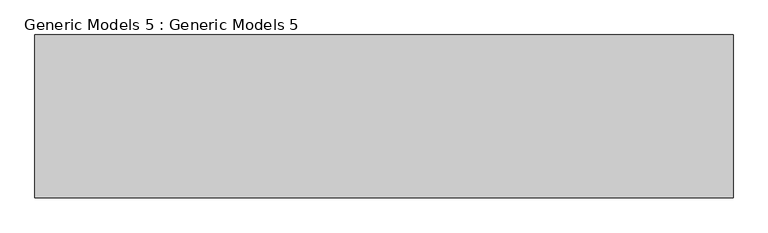
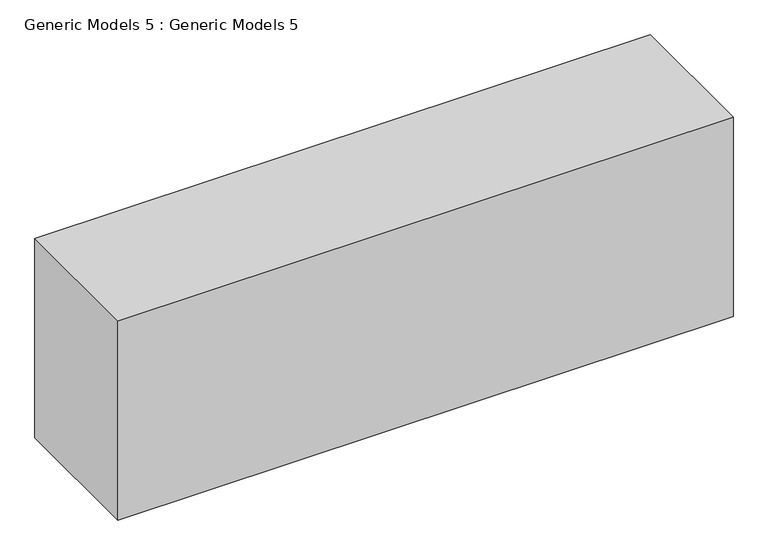
"""IFC4 building model written with IfcOpenShell, lengths in millimetres: proxy geometry, Generic Models 5 : Generic Models 5."""

from ifc_helpers import new_model, si_unit, frame, origin, place, context, project, spatial, polyline, outline, extrude, source, transform, mapped, element, save


def generic_models_5_generic_models_5_907641ea(model_context):
    return source(origin(), model_context, "Body", "SweptSolid", [
        extrude(outline(polyline([(52.3930105, -6017.2844717), (52.3930105, -7262.071797), (-5281.6069895, -7262.071797), (-5281.6069895, -6017.2844717), (52.3930105, -6017.2844717)])), frame((0.0, 0.0, 6400.8), z_axis=(0.0, 0.0, 1.0), x_axis=(1.0, 0.0, 0.0)), (0.0, 0.0, 1.0), 1828.8591279),
    ])


if __name__ == "__main__":
    model = new_model("IFC4")
    model_context = context("Model", 3, world=origin())
    ifc_project = project(units=[si_unit("LENGTHUNIT", "METRE", prefix="MILLI")], contexts=[model_context])
    site = spatial("IfcSite", under=ifc_project)
    building = spatial("IfcBuilding", under=site)
    placement = place(None, origin())
    generic_models_5_generic_models_5_shape = generic_models_5_generic_models_5_907641ea(model_context)
    element("IfcBuildingElementProxy", 1, Name="Generic Models 5 : Generic Models 5", ObjectType="Generic Models 5 : Generic Models 5", at=placement, inside=building, context=model_context, shape_type="MappedRepresentation", body=[
        mapped(generic_models_5_generic_models_5_shape, transform((0.0, 0.0, 0.0), x_axis=(1.0, 0.0, 0.0), y_axis=(0.0, 1.0, 0.0), z_axis=(0.0, 0.0, 1.0))),
    ])
    save(model, "model.ifc")
